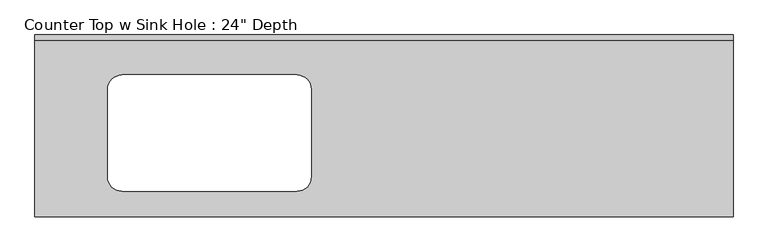
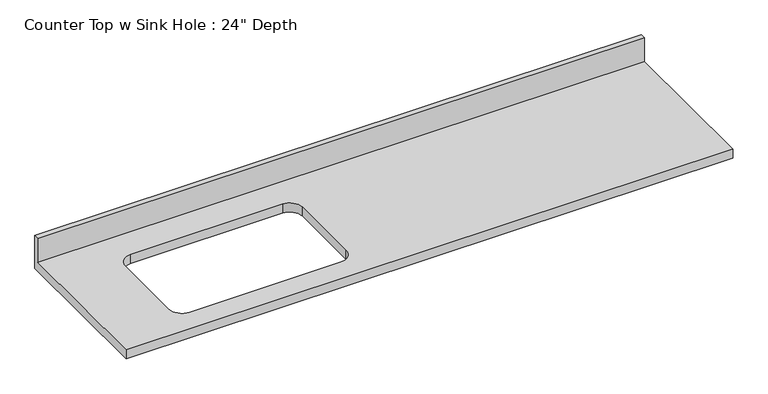
"""IFC4 building model written with IfcOpenShell, lengths in millimetres: furniture geometry."""

from ifc_helpers import new_model, si_unit, frame, origin, place, context, project, spatial, polyline, circle_curve, source, transform, mapped, element, save
from ifc_brep_helpers import plane_surface, revolved_surface, advanced_brep


def furniture_22cae41e(model_context):
    return source(origin(), model_context, "Body", "AdvancedBrep", [
        advanced_brep(
        [(-1200.4622951, -635.0, 914.4), (1237.9377049, -635.0, 914.4), (1237.9377049, -19.05, 914.4), (-1200.4622951, -19.05, 914.4), (-895.6622951, -139.7, 914.4), (-286.0622951, -139.7, 914.4), (-235.2622951, -190.5, 914.4), (-235.2622951, -495.3, 914.4), (-286.0622951, -546.1, 914.4), (-895.6622951, -546.1, 914.4), (-946.4622951, -495.3, 914.4), (-946.4622951, -190.5, 914.4), (1237.9377049, 0.0, 876.3), (1237.9377049, -635.0, 876.3), (-1200.4622951, -635.0, 876.3), (-1200.4622951, 0.0, 876.3), (-286.0622951, -139.7, 876.3), (-895.6622951, -139.7, 876.3), (-946.4622951, -190.5, 876.3), (-946.4622951, -495.3, 876.3), (-895.6622951, -546.1, 876.3), (-286.0622951, -546.1, 876.3), (-235.2622951, -495.3, 876.3), (-235.2622951, -190.5, 876.3), (-1200.4622951, 0.0, 1016.0), (1237.9377049, 0.0, 1016.0), (-1200.4622951, -19.05, 1016.0), (1237.9377049, -19.05, 1016.0)],
        [
            (0, 1),
            (1, 2),
            (2, 3),
            (3, 0),
            (4, 5),
            (5, 6, circle_curve(frame((-286.0622951, -190.5, 914.4), z_axis=(0.0, 0.0, -1.0), x_axis=(1.0, 0.0, 0.0)), 50.8)),
            (6, 7),
            (7, 8, circle_curve(frame((-286.0622951, -495.3, 914.4), z_axis=(0.0, 0.0, -1.0), x_axis=(1.0, 0.0, 0.0)), 50.8)),
            (8, 9),
            (9, 10, circle_curve(frame((-895.6622951, -495.3, 914.4), z_axis=(0.0, 0.0, -1.0), x_axis=(1.0, 0.0, 0.0)), 50.8)),
            (10, 11),
            (11, 4, circle_curve(frame((-895.6622951, -190.5, 914.4), z_axis=(0.0, 0.0, -1.0), x_axis=(1.0, 0.0, 0.0)), 50.8)),
            (12, 13),
            (13, 14),
            (14, 15),
            (15, 12),
            (16, 17),
            (17, 18, circle_curve(frame((-895.6622951, -190.5, 876.3), z_axis=(0.0, 0.0, 1.0), x_axis=(1.0, 0.0, 0.0)), 50.8)),
            (18, 19),
            (19, 20, circle_curve(frame((-895.6622951, -495.3, 876.3), z_axis=(0.0, 0.0, 1.0), x_axis=(1.0, 0.0, 0.0)), 50.8)),
            (20, 21),
            (21, 22, circle_curve(frame((-286.0622951, -495.3, 876.3), z_axis=(0.0, 0.0, 1.0), x_axis=(1.0, 0.0, 0.0)), 50.8)),
            (22, 23),
            (23, 16, circle_curve(frame((-286.0622951, -190.5, 876.3), z_axis=(0.0, 0.0, 1.0), x_axis=(1.0, 0.0, 0.0)), 50.8)),
            (15, 24),
            (24, 25),
            (25, 12),
            (14, 0),
            (3, 26),
            (26, 24),
            (13, 1),
            (25, 27),
            (27, 2),
            (26, 27),
            (4, 17),
            (16, 5),
            (11, 18),
            (10, 19),
            (9, 20),
            (8, 21),
            (7, 22),
            (6, 23),
        ],
        [
            plane_surface(frame((-1200.4622951, 0.0, 914.4), z_axis=(0.0, 0.0, 1.0), x_axis=(-1.0, 0.0, 0.0))),
            plane_surface(frame((-1200.4622951, 0.0, 876.3), z_axis=(0.0, 0.0, -1.0), x_axis=(1.0, 0.0, 0.0))),
            plane_surface(frame((1237.9377049, 0.0, 914.4), z_axis=(0.0, 1.0, 0.0), x_axis=(0.0, 0.0, -1.0))),
            plane_surface(frame((-1200.4622951, 0.0, 914.4), z_axis=(-1.0, 0.0, 0.0), x_axis=(0.0, 0.0, -1.0))),
            plane_surface(frame((-1200.4622951, -635.0, 914.4), z_axis=(0.0, -1.0, 0.0), x_axis=(0.0, 0.0, -1.0))),
            plane_surface(frame((1237.9377049, -635.0, 914.4), z_axis=(1.0, 0.0, 0.0), x_axis=(0.0, 0.0, -1.0))),
            plane_surface(frame((-1200.4622951, 0.0, 1016.0), z_axis=(0.0, 0.0, 1.0), x_axis=(0.0, -1.0, 0.0))),
            plane_surface(frame((-1200.4622951, -19.05, 1016.0), z_axis=(0.0, -1.0, 0.0), x_axis=(0.0, 0.0, -1.0))),
            plane_surface(frame((-286.0622951, -139.7, 914.4), z_axis=(0.0, -1.0, 0.0), x_axis=(0.0, 0.0, -1.0))),
            revolved_surface(polyline([(-844.8622951000001, -190.5, 914.4), (-844.8622951000001, -190.5, 876.3)]), (-895.6622951, -190.5, 876.3), (0.0, 0.0, 1.0)),
            plane_surface(frame((-946.4622951, -190.5, 914.4), z_axis=(1.0, 0.0, 0.0), x_axis=(0.0, 0.0, -1.0))),
            revolved_surface(polyline([(-844.8622951000001, -495.3, 914.4), (-844.8622951000001, -495.3, 876.3)]), (-895.6622951, -495.3, 876.3), (0.0, 0.0, 1.0)),
            plane_surface(frame((-895.6622951, -546.1, 914.4), z_axis=(0.0, 1.0, 0.0), x_axis=(0.0, 0.0, -1.0))),
            revolved_surface(polyline([(-235.26229509999996, -495.3, 914.4), (-235.26229509999996, -495.3, 876.3)]), (-286.0622951, -495.3, 876.3), (0.0, 0.0, 1.0)),
            plane_surface(frame((-235.2622951, -495.3, 914.4), z_axis=(-1.0, 0.0, 0.0), x_axis=(0.0, 0.0, -1.0))),
            revolved_surface(polyline([(-235.26229509999996, -190.5, 914.4), (-235.26229509999996, -190.5, 876.3)]), (-286.0622951, -190.5, 876.3), (0.0, 0.0, 1.0)),
        ],
        [
            (0, [[1, 2, 3, 4], [5, 6, 7, 8, 9, 10, 11, 12]]),
            (1, [[13, 14, 15, 16], [17, 18, 19, 20, 21, 22, 23, 24]]),
            (2, [[-16, 25, 26, 27]]),
            (3, [[-15, 28, -4, 29, 30, -25]]),
            (4, [[-1, -28, -14, 31]]),
            (5, [[-13, -27, 32, 33, -2, -31]]),
            (6, [[-30, 34, -32, -26]]),
            (7, [[-34, -29, -3, -33]]),
            (8, [[35, -17, 36, -5]]),
            (9, [[-35, -12, 37, -18]]),
            (10, [[-37, -11, 38, -19]]),
            (11, [[-38, -10, 39, -20]]),
            (12, [[-39, -9, 40, -21]]),
            (13, [[-40, -8, 41, -22]]),
            (14, [[-41, -7, 42, -23]]),
            (15, [[-36, -24, -42, -6]]),
        ],
    ),
    ])


if __name__ == "__main__":
    model = new_model("IFC4")
    model_context = context("Model", 3, world=origin())
    ifc_project = project(units=[si_unit("LENGTHUNIT", "METRE", prefix="MILLI")], contexts=[model_context])
    site = spatial("IfcSite", under=ifc_project)
    building = spatial("IfcBuilding", under=site)
    placement = place(None, origin())
    furniture_shape = furniture_22cae41e(model_context)
    element("IfcFurniture", 1, ObjectType="Counter Top w Sink Hole : 24\" Depth", at=placement, inside=building, context=model_context, shape_type="MappedRepresentation", body=[
        mapped(furniture_shape, transform((0.0, 0.0, 0.0), x_axis=(1.0, 0.0, 0.0), y_axis=(0.0, 1.0, 0.0), z_axis=(0.0, 0.0, 1.0))),
    ])
    save(model, "model.ifc")

# Revit data of these elements
# Type "Counter Top w Sink Hole : 24\" Depth"
#   Assembly Code = "C1030400"
#   Counter Thickness = 0' - 1 1/2"
#   Depth = 2' - 1"
#   Height = 3' - 0"
#   Length [instance default] = 8' - 0"
#   Sink Location [instance default] = 2' - 0"
#   Sink Location To Wall [instance default] = 0' - 6"
#   Sink Opening Depth [instance default] = 1' - 3"
#   Sink Opening Width [instance default] = 2' - 3"
#   Counter Top Material = none
#   Default Elevation = 0
# Element 1 (IfcFurniture, "Counter Top w Sink Hole : 24\" Depth")
#   Materials on its faces: "Counter Top"
# Materials
#   "Counter Top": class "Wood", colour RGB 226 177 128, transparency 0
